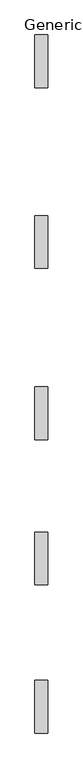
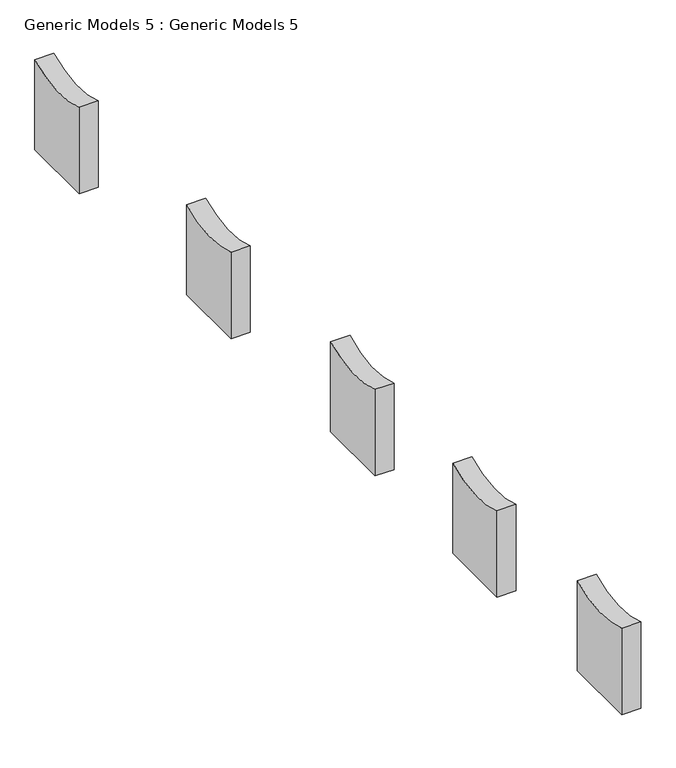
"""IFC4 building model written with IfcOpenShell, lengths in millimetres: proxy geometry, Generic Models 5 : Generic Models 5."""

from ifc_helpers import new_model, si_unit, point, frame, frame_2d, origin, place, context, project, spatial, polyline, circle_curve, trimmed, segment, composite_curve, outline, extrude, source, transform, mapped, element, save


def generic_models_5_generic_models_5_faea7b41(model_context):
    return source(origin(), model_context, "Body", "SweptSolid", [
        extrude(outline(composite_curve([segment(polyline([(-7377.644927, 812.8), (-7377.644927, 2275.3726309)]), True, "CONTINUOUS"), segment(trimmed(circle_curve(frame_2d((-6835.2291302, 3720.862745)), 1543.9095073), [point((-7377.644927, 2275.3726309))], [point((-6151.104226, 2336.8))], True, "CARTESIAN"), True, "CONTINUOUS"), segment(polyline([(-6151.104226, 2336.8), (-6151.104226, 812.8), (-7377.644927, 812.8)]), True, "CONTINUOUS")], self_intersect=False)), frame((-9446.2512244, 0.0, 0.0), z_axis=(1.0, 0.0, 0.0), x_axis=(0.0, 1.0, 0.0)), (0.0, 0.0, 1.0), 304.8),
        extrude(outline(composite_curve([segment(polyline([(-3926.6183645, 704.8336361), (-3926.6183645, 2167.406267)]), True, "CONTINUOUS"), segment(trimmed(circle_curve(frame_2d((-3384.2025677, 3612.8963811)), 1543.9095073), [point((-3926.6183645, 2167.406267))], [point((-2700.0776635, 2228.8336361))], True, "CARTESIAN"), True, "CONTINUOUS"), segment(polyline([(-2700.0776635, 2228.8336361), (-2700.0776635, 704.8336361), (-3926.6183645, 704.8336361)]), True, "CONTINUOUS")], self_intersect=False)), frame((-9446.2512244, 0.0, 0.0), z_axis=(1.0, 0.0, 0.0), x_axis=(0.0, 1.0, 0.0)), (0.0, 0.0, 1.0), 304.8),
        extrude(outline(composite_curve([segment(polyline([(-543.2589895, 704.8336361), (-543.2589895, 2167.406267)]), True, "CONTINUOUS"), segment(trimmed(circle_curve(frame_2d((-0.8431927, 3612.8963811)), 1543.9095073), [point((-543.2589895, 2167.406267))], [point((683.2817115, 2228.8336361))], True, "CARTESIAN"), True, "CONTINUOUS"), segment(polyline([(683.2817115, 2228.8336361), (683.2817115, 704.8336361), (-543.2589895, 704.8336361)]), True, "CONTINUOUS")], self_intersect=False)), frame((-9446.2512244, 0.0, 0.0), z_axis=(1.0, 0.0, 0.0), x_axis=(0.0, 1.0, 0.0)), (0.0, 0.0, 1.0), 304.8),
        extrude(outline(composite_curve([segment(polyline([(3449.105073, 603.2336361), (3449.105073, 2065.806267)]), True, "CONTINUOUS"), segment(trimmed(circle_curve(frame_2d((3991.5208698, 3511.2963811)), 1543.9095073), [point((3449.105073, 2065.806267))], [point((4675.645774, 2127.2336361))], True, "CARTESIAN"), True, "CONTINUOUS"), segment(polyline([(4675.645774, 2127.2336361), (4675.645774, 603.2336361), (3449.105073, 603.2336361)]), True, "CONTINUOUS")], self_intersect=False)), frame((-9446.2512244, 0.0, 0.0), z_axis=(1.0, 0.0, 0.0), x_axis=(0.0, 1.0, 0.0)), (0.0, 0.0, 1.0), 304.8),
        extrude(outline(composite_curve([segment(polyline([(7655.1110933, 501.6336361), (7655.1110933, 1964.206267)]), True, "CONTINUOUS"), segment(trimmed(circle_curve(frame_2d((8197.5268902, 3409.6963811)), 1543.9095073), [point((7655.1110933, 1964.206267))], [point((8881.6517944, 2025.6336361))], True, "CARTESIAN"), True, "CONTINUOUS"), segment(polyline([(8881.6517944, 2025.6336361), (8881.6517944, 501.6336361), (7655.1110933, 501.6336361)]), True, "CONTINUOUS")], self_intersect=False)), frame((-9446.2512244, 0.0, 0.0), z_axis=(1.0, 0.0, 0.0), x_axis=(0.0, 1.0, 0.0)), (0.0, 0.0, 1.0), 304.8),
    ])


if __name__ == "__main__":
    model = new_model("IFC4")
    model_context = context("Model", 3, world=origin())
    ifc_project = project(units=[si_unit("LENGTHUNIT", "METRE", prefix="MILLI")], contexts=[model_context])
    site = spatial("IfcSite", under=ifc_project)
    building = spatial("IfcBuilding", under=site)
    placement = place(None, origin())
    generic_models_5_generic_models_5_shape = generic_models_5_generic_models_5_faea7b41(model_context)
    element("IfcBuildingElementProxy", 1, Name="Generic Models 5 : Generic Models 5", ObjectType="Generic Models 5 : Generic Models 5", at=placement, inside=building, context=model_context, shape_type="MappedRepresentation", body=[
        mapped(generic_models_5_generic_models_5_shape, transform((0.0, 0.0, 0.0), x_axis=(1.0, 0.0, 0.0), y_axis=(0.0, 1.0, 0.0), z_axis=(0.0, 0.0, 1.0))),
    ])
    save(model, "model.ifc")

# Revit data of these elements
# Element 1 (IfcBuildingElementProxy, "Generic Models 5 : Generic Models 5")
#   Materials on its faces: "Parking Stripe"
# Materials
#   "Parking Stripe": class "Paint", colour RGB 250 250 91, transparency 0, Cost = 0
